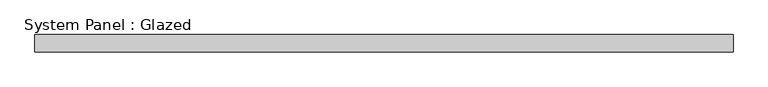
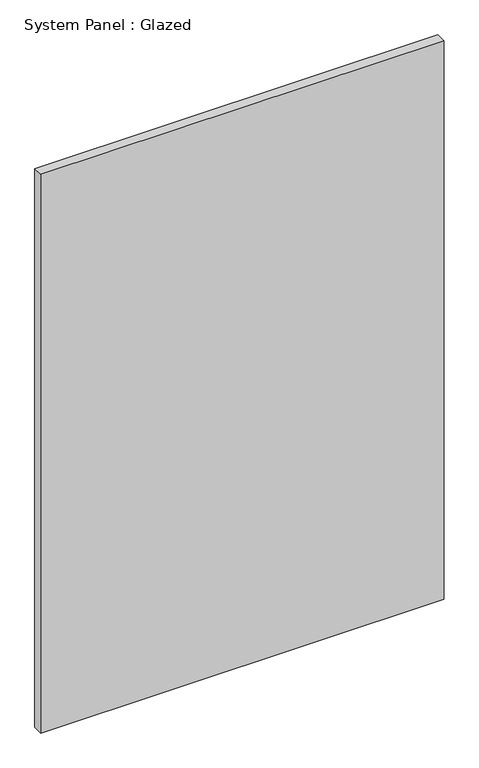
"""IFC4 building model written with IfcOpenShell, lengths in millimetres: plate geometry, System Panel : Glazed."""

from ifc_helpers import new_model, si_unit, origin, origin_with_axes, place, context, project, spatial, polyline, outline, extrude, source, transform, mapped, element, save


def system_panel_glazed_8ae820b6(model_context):
    return source(origin(), model_context, "Body", "SweptSolid", [
        extrude(outline(polyline([(517.525, 19.05), (-517.525, 19.05), (-517.525, 44.45), (517.525, 44.45), (517.525, 19.05)])), origin_with_axes(), (0.0, 0.0, 1.0), 1515.7479304),
    ])


if __name__ == "__main__":
    model = new_model("IFC4")
    model_context = context("Model", 3, world=origin())
    ifc_project = project(units=[si_unit("LENGTHUNIT", "METRE", prefix="MILLI")], contexts=[model_context])
    site = spatial("IfcSite", under=ifc_project)
    building = spatial("IfcBuilding", under=site)
    placement = place(None, origin())
    system_panel_glazed_shape = system_panel_glazed_8ae820b6(model_context)
    element("IfcPlate", 1, ObjectType="System Panel : Glazed", at=placement, inside=building, context=model_context, shape_type="MappedRepresentation", body=[
        mapped(system_panel_glazed_shape, transform((0.0, 0.0, 0.0), x_axis=(1.0, 0.0, 0.0), y_axis=(0.0, 1.0, 0.0), z_axis=(0.0, 0.0, 1.0))),
    ])
    save(model, "model.ifc")

# Revit data of these elements
# Type "System Panel : Glazed"
#   Construction Type Id = "GSP4R"
#   Analytic Construction = "1/8 in Pilkington single glazing"
#   Visual Light Transmittance = 0.9
#   Solar Heat Gain Coefficient = 0.86
#   Heat Transfer Coefficient (U) = 1.18115 BTU/(h·ft²·°F)
#   Define Thermal Properties by = 1
# Element 1 (IfcPlate, "System Panel : Glazed")
#   Materials on its faces: "Glass"
# Materials
#   "Glass": class "Glass", colour RGB 0 128 192, transparency 0.75, Description = "Soda Lime Glass", Cost = 0
